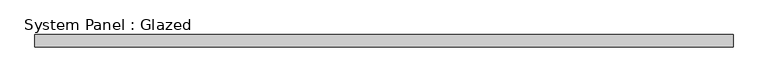
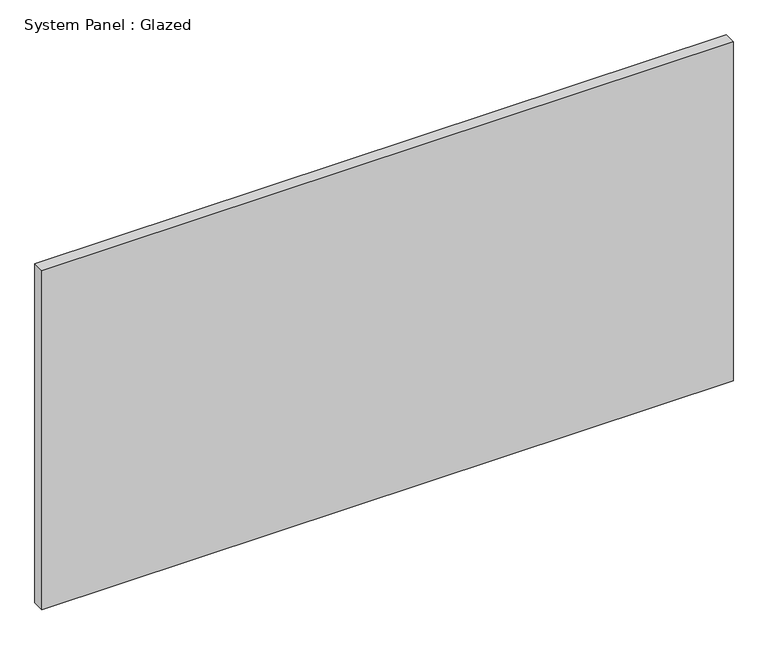
"""IFC4 building model written with IfcOpenShell, lengths in millimetres: plate geometry, System Panel : Glazed."""

from ifc_helpers import new_model, si_unit, origin, origin_with_axes, place, context, project, spatial, polyline, outline, extrude, source, transform, mapped, element, save


def system_panel_glazed_0d05c03e(model_context):
    return source(origin(), model_context, "Body", "SweptSolid", [
        extrude(outline(polyline([(730.25, 19.05), (-730.25, 19.05), (-730.25, 44.45), (730.25, 44.45), (730.25, 19.05)])), origin_with_axes(), (0.0, 0.0, 1.0), 757.5270145),
    ])


if __name__ == "__main__":
    model = new_model("IFC4")
    model_context = context("Model", 3, world=origin())
    ifc_project = project(units=[si_unit("LENGTHUNIT", "METRE", prefix="MILLI")], contexts=[model_context])
    site = spatial("IfcSite", under=ifc_project)
    building = spatial("IfcBuilding", under=site)
    placement = place(None, origin())
    system_panel_glazed_shape = system_panel_glazed_0d05c03e(model_context)
    element("IfcPlate", 1, ObjectType="System Panel : Glazed", at=placement, inside=building, context=model_context, shape_type="MappedRepresentation", body=[
        mapped(system_panel_glazed_shape, transform((0.0, 0.0, 0.0), x_axis=(1.0, 0.0, 0.0), y_axis=(0.0, 1.0, 0.0), z_axis=(0.0, 0.0, 1.0))),
    ])
    save(model, "model.ifc")

# Revit data of these elements
# Type "System Panel : Glazed"
#   Construction Type Id = "GSP4R"
#   Analytic Construction = "1/8 in Pilkington single glazing"
#   Visual Light Transmittance = 0.9
#   Solar Heat Gain Coefficient = 0.86
#   Heat Transfer Coefficient (U) = 1.18115 BTU/(h·ft²·°F)
#   Define Thermal Properties by = 1
# Element 1 (IfcPlate, "System Panel : Glazed")
#   Materials on its faces: "Glass"
# Materials
#   "Glass": class "Glass", colour RGB 0 128 192, transparency 0.75, Description = "Soda Lime Glass", Cost = 0
